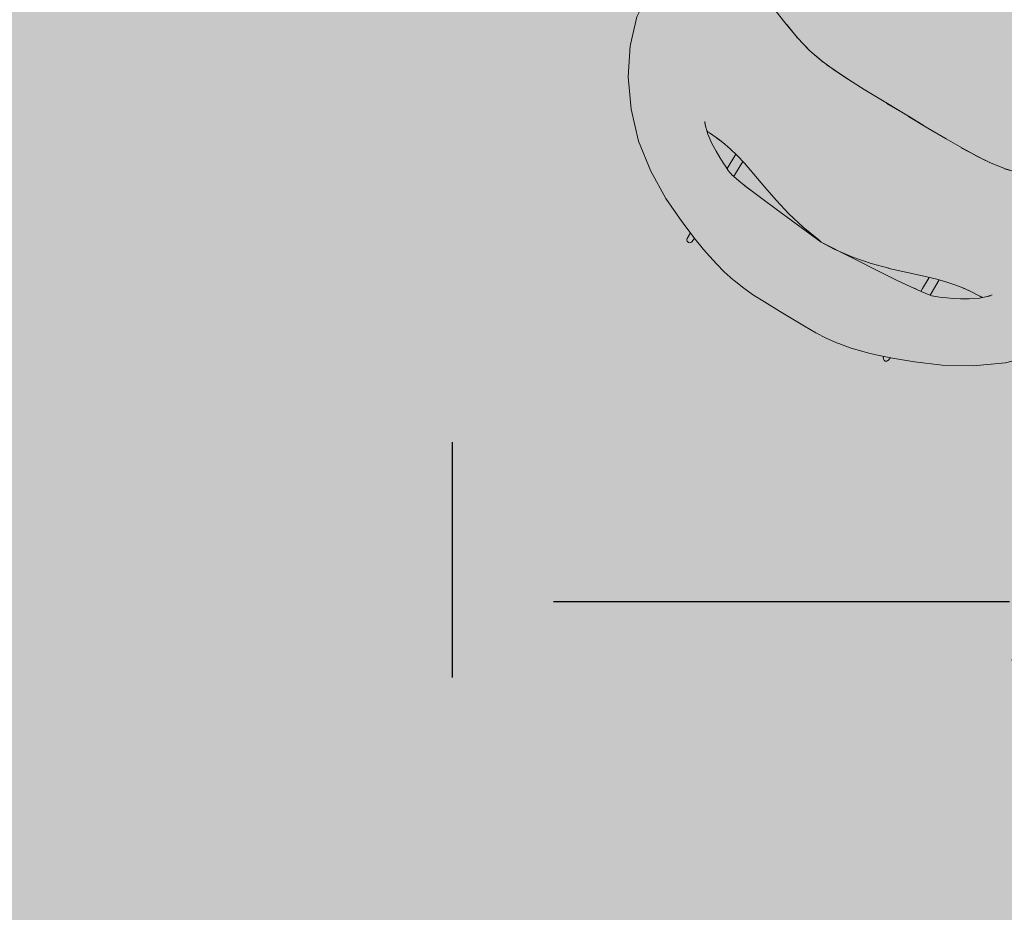
# Model space of a CAD drawing. Units: inches. Extents: x -466983 to 1020, y 324 to 318697.
# Tile 11 of 97: x 736 to 775, y 417 to 452. Entities that reach past the tile are written whole.
import ezdxf

# ---------------------------------------------------------------- set-up
doc = ezdxf.new("R2010")
doc.units = ezdxf.units.IN
doc.header["$MEASUREMENT"] = 0
for name, color, linetype, lineweight in [('A-ANNO-DIMS', 2, 'Continuous', 18), ('A-FLOR-PATT', 252, 'Continuous', 13), ('A-FURN', 8, 'Continuous', 18)]:
    doc.layers.add(name, color=color, linetype=linetype, lineweight=lineweight)
doc.layers.add('K-Hatch', color=7, linetype='Continuous')
doc.styles.get("Standard").update_dxf_attribs({"font": 'arial.ttf'})
doc.dimstyles.get("Standard").update_dxf_attribs({"dimtxt": 6, "dimasz": 4, "dimexe": 3, "dimexo": 3, "dimgap": 0.09, "dimtad": 0, "dimtih": 1, "dimtoh": 1, "dimdec": 1, "dimzin": 0, "dimdsep": 46, "dimlunit": 3, "dimtxsty": 'Standard', "dimcen": 0.09, "dimadec": 0, "dimazin": 0, "dimtfac": 1, "dimtdec": 1, "dimtofl": 0, "dimtmove": 0, "dimatfit": 3, "dimfxl": 1, "dimtolj": 1, "dimtzin": 0, "dimarcsym": 0})

# ---------------------------------------------------------------- blocks, each defined once
blk = doc.blocks.new('CBV_06')
at = {"layer": 'K-Hatch'}
h = blk.add_hatch(color=256, dxfattribs=at)
h.dxf.hatch_style = 1
h.paths.add_polyline_path([(1007.6, -162.8), (976.4, -65), (974.5, -60.9), (923.4, 38), (854.3, 132.5), (771.1, 217.3), (677.3, 287), (580.7, 342.5), (489.2, 384.4), (414.7, 413.4), (369.4, 429.9), (337.4, 440.2), (302.9, 450.6), (264.8, 460.4), (221.9, 468.5), (217.5, 469.1), (173.4, 474.9), (131.2, 477.6), (84.4, 478.5), (-21.2, 478.6), (-84.4, 478.5), (-131.2, 477.6), (-173.4, 474.9), (-217.5, 469.1), (-221.9, 468.5), (-264.8, 460.4), (-302.9, 450.6), (-337.4, 440.2), (-369.4, 429.9), (-414.7, 413.4), (-489.2, 384.4), (-580.7, 342.5), (-677.3, 287), (-771.1, 217.3), (-854.3, 132.5), (-923.4, 38), (-974.5, -60.9), (-976.4, -65), (-1007.6, -162.8), (-1016.4, -252), (-1016.2, -257.5), (-1002.7, -333.7), (-999.3, -339.8), (-963.8, -397.3), (-956.9, -403.9), (-946.2, -410.9), (-945.1, -411.6), (-892.7, -445.8), (-879.3, -451.9), (-863.7, -457.7), (-847.5, -463.3), (-832.6, -467.9), (-820.8, -470.9), (-811.5, -472.7), (-749.7, -478.5), (-742.9, -478.6), (-675.1, -467.1), (-608, -445.9), (-540.7, -420.5), (-533.5, -417.9), (-475.1, -397.7), (-450.5, -390.8), (-411.1, -379.9), (-386, -375.8), (-353.2, -370.6), (-333.2, -368.9), (-297.7, -366.2), (-239.9, -363.6), (-171.9, -362.2), (-95.5, -361.3), (-76.2, -361.4), (-13.7, -361.6), (-21.2, -361.9), (13.7, -361.6), (76.2, -361.4), (95.5, -361.3), (171.9, -362.2), (239.9, -363.6), (297.7, -366.2), (333.2, -368.9), (353.2, -370.6), (386, -375.8), (411.1, -379.9), (450.4, -390.7), (475.1, -397.7), (533.4, -417.9), (540.7, -420.5), (608, -445.9), (675.1, -467.1), (742.9, -478.6), (749.7, -478.5), (811.5, -472.7), (820.8, -470.9), (832.6, -467.9), (847.5, -463.3), (863.7, -457.7), (879.3, -451.9), (892.7, -445.8), (945.1, -411.6), (946.2, -410.9), (956.9, -403.9), (963.8, -397.3), (999.3, -339.8), (1002.7, -333.7), (1016.2, -257.5), (1016.4, -252)])
h.paths.add_polyline_path([(474.4, 70.2), (440.8, 77.6), (404.4, 87.8), (354.2, 104.4), (296.4, 124), (237, 143.3), (236.1, 143.6), (173.2, 161.3), (104.7, 175.8), (50.1, 183.8), (-6.2, 188), (-21.2, 188.7), (-32.5, 186.3), (-104.7, 175.8), (-173.2, 161.3), (-236.1, 143.6), (-237, 143.3), (-296.4, 124), (-354.2, 104.4), (-404.4, 87.8), (-440.8, 77.6), (-474.4, 70.2), (-510.8, 64.3), (-524, 62.5), (-568.6, 59.8), (-577.9, 60.2), (-570.8, 66.8), (-541.1, 87.8), (-513.8, 104.1), (-490.9, 116.3), (-470.5, 126.5), (-453.3, 134.6), (-440.4, 140.4), (-432.6, 143.7), (-427.3, 145.8), (-423.1, 147.3), (-410.5, 149.9), (-379.3, 154.4), (-338.7, 159.3), (-285, 164.8), (-220.8, 170.8), (-21.2, 189.2), (-6.2, 188), (32.5, 186.3), (50.1, 183.8), (220.8, 170.8), (285, 164.8), (338.8, 159.3), (379.3, 154.4), (410.5, 149.9), (423.1, 147.3), (427.3, 145.8), (432.6, 143.7), (440.4, 140.4), (453.3, 134.6), (470.5, 126.5), (490.9, 116.3), (513.8, 104.1), (541.1, 87.8), (570.8, 66.8), (577.9, 60.2), (568.6, 59.8), (524, 62.5), (510.8, 64.3)], flags=16)
h = blk.add_hatch(color=256, dxfattribs=at)
h.dxf.hatch_style = 1
h.paths.add_polyline_path([(-412.4, 142.8), (-412.6, 149.4), (-423.1, 147.3), (-427.3, 145.8), (-432.6, 143.7), (-440.4, 140.4), (-447.9, 137), (-448.1, 76), (-440.8, 77.6), (-412.2, 85.6)])
h.paths.add_polyline_path([(413.4, 142.6), (413.2, 149.3), (410.5, 149.9), (379.3, 154.4), (378.3, 154.5), (378, 142.6), (377.8, 96.6), (404.4, 87.8), (413.6, 85.2)])
h.paths.add_polyline_path([(405.3, 429.7), (403.3, 432.8), (400.8, 434.7), (397.7, 435.9), (397.4, 435.9), (396.7, 435.9), (395.7, 435.9), (394.7, 435.9), (393.7, 435.9), (390.6, 434.7), (388.1, 432.8), (386.1, 429.7), (384.7, 426.5), (384.7, 424.3), (406.7, 416.3), (406.6, 426.5)])
h.paths.add_polyline_path([(-419.2, 426.7), (-420.5, 429.9), (-422.5, 433), (-425.1, 434.9), (-428.2, 436.2), (-428.4, 436.2), (-429.1, 436.2), (-430.1, 436.2), (-431.1, 436.2), (-432.1, 436.2), (-435.2, 434.9), (-437.7, 433), (-439.8, 429.9), (-441.1, 426.7), (-441.3, 403), (-419.1, 411.7)])
h = blk.add_hatch(color=256, dxfattribs=at)
h.dxf.hatch_style = 1
h.paths.add_polyline_path([(-296.4, 124), (-236.3, 143.6), (-173.2, 161.3), (-104.7, 175.8), (-32.5, 186.3), (-19.6, 189.1), (-21.2, 189.2), (-220.8, 170.8), (-285, 164.8), (-338.2, 159.4), (-360.5, 156.7), (-379.3, 154.4), (-410.5, 149.9), (-412.6, 149.4), (-412.4, 142.8), (-412.2, 85.6), (-404.4, 87.8), (-354.2, 104.4)])
h.paths.add_polyline_path([(-447.9, 137), (-453.3, 134.6), (-470.5, 126.5), (-490.9, 116.3), (-513.8, 104.1), (-541.1, 87.8), (-570.8, 66.8), (-577.9, 60.2), (-568.6, 59.8), (-535.5, 61.8), (-514.8, 63.7), (-510.8, 64.3), (-474.4, 70.2), (-448.1, 76)])
h = blk.add_hatch(color=256, dxfattribs=at)
h.dxf.hatch_style = 1
h.paths.add_polyline_path([(378, 142.6), (377.8, 96.6), (354.2, 104.4), (296.4, 124), (237, 143.3), (236.1, 143.6), (173.2, 161.3), (104.7, 175.8), (50.1, 183.8), (-6.2, 188), (-21.2, 188.7), (-32.5, 186.3), (-104.7, 175.8), (-173.2, 161.3), (-236.3, 143.6), (-237, 143.3), (-236.1, 143.6), (-173.2, 161.3), (-104.7, 175.8), (-32.5, 186.3), (-19.6, 189.1), (-6.2, 188), (32.5, 186.3), (50.1, 183.8), (220.8, 170.8), (285, 164.8), (338.8, 159.3), (378.3, 154.5)])
h.paths.add_polyline_path([(541.1, 87.8), (513.8, 104.1), (490.9, 116.3), (470.5, 126.5), (453.3, 134.6), (440.4, 140.4), (432.6, 143.7), (427.3, 145.8), (423.1, 147.3), (413.2, 149.3), (413.4, 142.6), (413.6, 85.2), (440.8, 77.6), (474.4, 70.2), (510.8, 64.3), (514.8, 63.7), (535.5, 61.8), (568.6, 59.8), (577.9, 60.2), (570.8, 66.8)])
for points in [[(472.3, -396.2), (540.7, -420.5), (608, -445.9), (675.1, -467.1), (742.9, -478.6), (749.7, -478.5), (811.5, -472.7), (820.8, -470.9), (832.6, -467.9), (847.5, -463.3), (863.7, -457.7), (879.3, -451.9), (892.7, -445.8), (946.2, -410.9), (956.9, -403.9), (963.8, -397.3), (999.3, -339.8), (1002.7, -333.7), (1016.2, -257.5), (1016.4, -252), (1007.6, -162.8), (976.4, -65), (974.5, -60.9), (923.4, 38), (854.3, 132.5), (771.1, 217.3), (677.3, 287), (580.7, 342.5), (489.2, 384.4), (414.7, 413.4), (369.4, 429.9), (337.4, 440.2), (302.9, 450.6), (264.8, 460.4), (221.9, 468.5), (217.5, 469.1), (173.4, 474.9), (131.2, 477.6), (84.4, 478.5), (-21.2, 478.6), (-84.4, 478.5), (-131.2, 477.6), (-173.4, 474.9), (-217.5, 469.1), (-221.9, 468.5), (-264.8, 460.4), (-302.9, 450.6), (-337.4, 440.2), (-369.4, 429.9), (-414.7, 413.4), (-489.2, 384.4), (-580.7, 342.5), (-677.3, 287), (-771.1, 217.3), (-854.3, 132.5), (-923.4, 38), (-974.5, -60.9), (-976.4, -65), (-1007.6, -162.8), (-1016.4, -252), (-1016.2, -257.5), (-1002.7, -333.7), (-999.3, -339.8), (-963.8, -397.3), (-956.9, -403.9), (-946.2, -410.9), (-892.7, -445.8), (-879.3, -451.9), (-863.7, -457.7), (-847.5, -463.3), (-832.6, -467.9), (-820.8, -470.9), (-811.5, -472.7), (-749.7, -478.5), (-742.9, -478.6), (-675.1, -467.1), (-608, -445.9), (-540.7, -420.5), (-472.3, -396.2)], [(-441.3, 403), (-441.1, 426.7), (-439.8, 429.9), (-437.7, 433), (-435.2, 434.9), (-432.1, 436.2), (-431.9, 436.2), (-431.1, 436.2), (-430.1, 436.2), (-429.1, 436.2), (-428.4, 436.2), (-428.2, 436.2), (-425.1, 434.9), (-422.5, 433), (-420.5, 429.9), (-419.2, 426.7), (-419.1, 411.7)], [(384.7, 424.3), (384.7, 426.5), (386.1, 429.7), (388.1, 432.8), (390.6, 434.7), (393.7, 435.9), (394, 435.9), (394.7, 435.9), (395.7, 435.9), (396.7, 435.9), (397.4, 435.9), (397.7, 435.9), (400.8, 434.7), (403.3, 432.8), (405.3, 429.7), (406.6, 426.5), (406.7, 416.3)], [(-510.8, 64.3), (-474.4, 70.2), (-440.8, 77.6), (-404.4, 87.8), (-354.2, 104.4), (-296.4, 124), (-237, 143.3), (-236.1, 143.6), (-173.2, 161.3), (-104.7, 175.8), (-32.5, 186.3), (-21.2, 188.7), (32.5, 186.3), (104.7, 175.8), (173.2, 161.3), (236.1, 143.6), (237, 143.3), (296.4, 124), (354.2, 104.4), (404.4, 87.8), (440.8, 77.6), (474.4, 70.2), (510.8, 64.3)], [(360.5, 156.7), (338.2, 159.4), (285, 164.8), (220.8, 170.8), (-21.2, 189.2), (-220.8, 170.8), (-285, 164.8), (-338.2, 159.4), (-360.5, 156.7)], [(-421.5, 147.9), (-427.3, 145.8), (-432.6, 143.7), (-440.4, 140.4), (-453.3, 134.6), (-470.5, 126.5), (-490.9, 116.3), (-513.8, 104.1), (-541.1, 87.8), (-570.8, 66.8), (-600.5, 39.3)], [(-335.3, 159.7), (-379.3, 154.4), (-410.5, 149.9), (-423.1, 147.3)], [(-412.6, 149.4), (-412.4, 142.8), (-412.2, 85.6)], [(423.1, 147.3), (410.5, 149.9), (379.3, 154.4), (335.3, 159.7)], [(377.8, 96.6), (378, 142.6), (378.3, 154.5)], [(413.2, 149.3), (413.4, 142.6), (413.6, 85.2)], [(600.5, 39.3), (570.8, 66.8), (541.1, 87.8), (513.8, 104.1), (490.9, 116.3), (470.5, 126.5), (453.3, 134.6), (440.4, 140.4), (432.6, 143.7), (427.3, 145.8), (421.5, 147.9)], [(-448.1, 76), (-447.9, 137)], [(-440.6, 77.6), (-440.8, 77.6)], [(440.8, 77.6), (440.8, 77.6)], [(-592.1, 47.1), (-604, 32.8)], [(-578.8, 59.3), (-575, 58.9)], [(-577.9, 60.2), (-568.6, 59.8), (-524, 62.5), (-499.7, 65.8)], [(-514.8, 63.7), (-535.5, 61.8)], [(499.7, 65.8), (524, 62.5), (568.6, 59.8), (577.9, 60.2)], [(535.5, 61.8), (514.8, 63.7)], [(575, 58.9), (578.8, 59.3)], [(604, 32.8), (592.1, 47.1)], [(-533.4, -417.9), (-475.1, -397.7), (-408.3, -378.8)], [(-450.4, -390.7), (-411.1, -379.9), (-350, -369.8)], [(-385.9, -375.7), (-353.2, -370.6), (-293.7, -365.6)], [(-333.2, -368.9), (-297.2, -366.2), (-234.6, -362.7)], [(-297.7, -366.2), (-239.9, -363.6), (-171.9, -362.2), (-95.5, -361.3), (-14.3, -361.4)], [(-76.4, -361.4), (-13.7, -361.6), (-21.2, -361.9), (13.7, -361.6), (76.4, -361.4)], [(14.3, -361.4), (95.5, -361.3), (171.9, -362.2), (239.9, -363.6), (297.7, -366.2)], [(234.7, -362.7), (297.2, -366.2), (333.2, -368.9)], [(293.7, -365.6), (353.2, -370.6), (385.9, -375.7)], [(350, -369.8), (411.1, -379.9), (450.4, -390.7)], [(408.3, -378.8), (475.1, -397.7), (533.4, -417.9)], [(-892.7, -445.8), (-902.5, -439.6), (-946.2, -410.9), (-956.9, -403.9)], [(892.7, -445.8), (902.5, -439.6), (946.2, -410.9), (956.9, -403.9)]]:
    blk.add_lwpolyline(points)
blk = doc.blocks.new('Garden Sofa')
at = {"xscale": -0.0109740885734132, "yscale": 0.0109740885734132, "zscale": 0.0109740885734132, "rotation": 148.8828363109627}
blk.add_blockref('CBV_06', (2441.681, 808.037), dxfattribs=at)
blk = doc.blocks.new('*D94')
at = {"layer": 'A-ANNO-DIMS', "color": 0, "lineweight": -2, "transparency": 16777216}
for p, q in [((753.135, 435.777), (753.135, 426.477)), ((805.966, 435.777), (805.966, 426.477)), ((757.135, 429.477), (775.163, 429.477)), ((801.966, 429.477), (783.938, 429.477))]:
    blk.add_line(p, q, dxfattribs=at)
at = {"layer": 'A-ANNO-DIMS', "color": 0, "transparency": 16777216}
for points in [[(757.135, 430.143), (757.135, 428.81), (753.135, 429.477)], [(801.966, 430.143), (801.966, 428.81), (805.966, 429.477)]]:
    blk.add_solid(points, dxfattribs=at)
at = {"layer": 'Defpoints', "color": 0, "transparency": 16777216}
for p in [(753.135, 438.777), (805.966, 438.777), (805.966, 429.477)]:
    blk.add_point(p, dxfattribs=at)
at = {"layer": 'A-ANNO-DIMS', "color": 0, "transparency": 16777216, "insert": (779.551, 429.477), "char_height": 6, "attachment_point": 5}
blk.add_mtext('\\A1;53', dxfattribs=at)

msp = doc.modelspace()

# ---------------------------------------------------------------- hatches: boundary and pattern name
at = {"layer": 'A-FLOR-PATT', "transparency": 33554661}
h = msp.add_hatch(color=256, dxfattribs=at)
h.dxf.hatch_style = 1
h.set_gradient(color1=(19, 155, 72), color2=(0, 107, 0), name='CYLINDER')
h.paths.add_polyline_path([(813.806, 503.938), (730.806, 503.938), (730.806, 424.938), (612.806, 424.938), (612.806, 415.938), (442.806, 415.938), (442.806, 368.938), (813.806, 368.938)])
h.paths.add_polyline_path([(771.796, 407.07), (783.796, 407.07), (783.796, 371.07), (771.796, 371.07)], flags=16)
h.paths.add_polyline_path([(755.796, 407.07), (755.796, 371.07), (743.796, 371.07), (743.796, 407.07)], flags=16)
h.paths.add_polyline_path([(769.796, 404.07), (769.796, 374.07), (757.796, 374.07), (757.796, 404.07)], flags=16)
h.paths.add_polyline_path([(785.796, 404.07), (797.796, 404.07), (797.796, 374.07), (785.796, 374.07)], flags=16)
h.paths.add_polyline_path([(741.796, 404.07), (741.796, 374.07), (729.796, 374.07), (729.796, 404.07)], flags=16)
h.paths.add_polyline_path([(799.796, 407.07), (811.796, 407.07), (811.796, 371.07), (799.796, 371.07)], flags=16)
h.paths.add_polyline_path([(727.796, 407.07), (727.796, 371.07), (715.796, 371.07), (715.796, 407.07)], flags=16)
h.paths.add_polyline_path([(713.796, 404.07), (713.796, 374.07), (701.796, 374.07), (701.796, 404.07)], flags=16)
h.paths.add_polyline_path([(699.796, 407.07), (699.796, 371.07), (687.796, 371.07), (687.796, 407.07)], flags=16)
h.paths.add_polyline_path([(685.796, 404.07), (685.796, 374.07), (673.796, 374.07), (673.796, 404.07)], flags=16)
h.paths.add_polyline_path([(671.796, 407.07), (671.796, 371.07), (659.796, 371.07), (659.796, 407.07)], flags=16)
h.paths.add_polyline_path([(657.796, 404.07), (657.796, 374.07), (645.796, 374.07), (645.796, 404.07)], flags=16)
h.paths.add_polyline_path([(643.796, 407.07), (643.796, 371.07), (631.796, 371.07), (631.796, 407.07)], flags=16)
h.paths.add_polyline_path([(629.796, 404.07), (629.796, 374.07), (617.796, 374.07), (617.796, 404.07)], flags=16)
h.paths.add_polyline_path([(615.796, 407.07), (615.796, 371.07), (603.796, 371.07), (603.796, 407.07)], flags=16)
h.paths.add_polyline_path([(601.796, 404.07), (601.796, 374.07), (589.796, 374.07), (589.796, 404.07)], flags=16)
at = {"layer": 'A-FLOR-PATT'}
h = msp.add_hatch(dxfattribs=at)
h.set_pattern_fill('GRASS', color=256, scale=6)
h.set_pattern_definition([(90, (-1212.4137, -290.035), (-4.242641, 4.242641), [1.125, -7.360281]), (45, (-1212.4137, -290.035), (-4.24264, 4.24264), [1.125, -4.875]), (135, (-1212.4137, -290.035), (-4.24264, -4.24264), [1.125, -4.875])])
h.paths.add_polyline_path([(813.806, 503.938), (730.806, 503.938), (730.806, 424.938), (612.806, 424.938), (612.806, 415.938), (442.806, 415.938), (442.806, 368.938), (813.806, 368.938)])
h.paths.add_polyline_path([(589.796, 404.07), (601.796, 404.07), (601.796, 374.07), (589.796, 374.07)], flags=16)
h.paths.add_polyline_path([(603.796, 407.07), (615.796, 407.07), (615.796, 371.07), (603.796, 371.07)], flags=16)
h.paths.add_polyline_path([(617.796, 404.07), (629.796, 404.07), (629.796, 374.07), (617.796, 374.07)], flags=16)
h.paths.add_polyline_path([(631.796, 407.07), (643.796, 407.07), (643.796, 371.07), (631.796, 371.07)], flags=16)
h.paths.add_polyline_path([(645.796, 404.07), (657.796, 404.07), (657.796, 374.07), (645.796, 374.07)], flags=16)
h.paths.add_polyline_path([(659.796, 407.07), (671.796, 407.07), (671.796, 371.07), (659.796, 371.07)], flags=16)
h.paths.add_polyline_path([(673.796, 404.07), (685.796, 404.07), (685.796, 374.07), (673.796, 374.07)], flags=16)
h.paths.add_polyline_path([(687.796, 407.07), (699.796, 407.07), (699.796, 371.07), (687.796, 371.07)], flags=16)
h.paths.add_polyline_path([(701.796, 404.07), (713.796, 404.07), (713.796, 374.07), (701.796, 374.07)], flags=16)
h.paths.add_polyline_path([(715.796, 407.07), (727.796, 407.07), (727.796, 371.07), (715.796, 371.07)], flags=16)
h.paths.add_polyline_path([(729.796, 404.07), (741.796, 404.07), (741.796, 374.07), (729.796, 374.07)], flags=16)
h.paths.add_polyline_path([(743.796, 407.07), (755.796, 407.07), (755.796, 371.07), (743.796, 371.07)], flags=16)
h.paths.add_polyline_path([(757.796, 404.07), (769.796, 404.07), (769.796, 374.07), (757.796, 374.07)], flags=16)
h.paths.add_polyline_path([(771.796, 407.07), (783.796, 407.07), (783.796, 371.07), (771.796, 371.07)], flags=16)
h.paths.add_polyline_path([(785.796, 404.07), (797.796, 404.07), (797.796, 374.07), (785.796, 374.07)], flags=16)
h.paths.add_polyline_path([(799.796, 407.07), (811.796, 407.07), (811.796, 371.07), (799.796, 371.07)], flags=16)

# ---------------------------------------------------------------- block references
at = {"layer": 'A-FURN'}
msp.add_blockref('Garden Sofa', (-1672.7, -362.711), dxfattribs=at)

# ---------------------------------------------------------------- dimensions: what is measured, and where the dimension line sits
at = {"layer": 'A-ANNO-DIMS'}
dim = msp.add_linear_dim(base=(805.966, 429.477), p1=(753.135, 438.777), p2=(805.966, 438.777), dimstyle='Standard', override={"dimdec": 0, "dimlfac": 1, "dimrnd": 0, "dimzin": 0, "dimdsep": 46, "dimlunit": 2}, dxfattribs=at)
dim.commit()
dim.dimension.update_dxf_attribs({"geometry": '*D94', "text_midpoint": (779.551, 429.477)})

doc.saveas('drawing.dxf')
